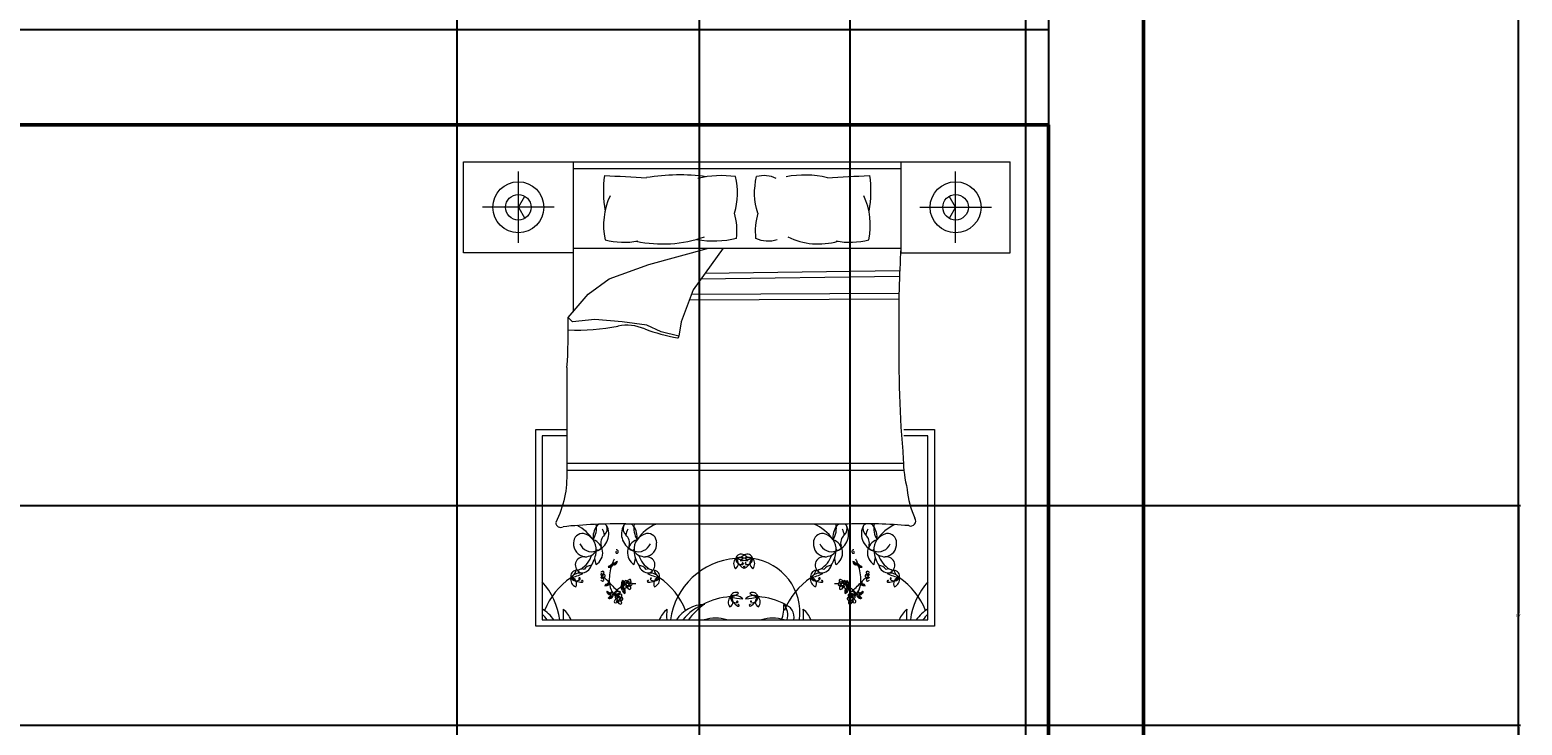
# Model space of a CAD drawing. Units: inches. Extents: x 3 to 576, y -689 to 51.
# Tile 11 of 21: x 435 to 576, y -506 to -440. Entities that reach past the tile are written whole.
import ezdxf

# ---------------------------------------------------------------- set-up
doc = ezdxf.new("R2010")
doc.units = ezdxf.units.IN
doc.header["$MEASUREMENT"] = 0
for name, color, linetype, lineweight in [('A-ANNO-DIMS', 2, 'Continuous', 18), ('A-FURN', 8, 'Continuous', 18), ('A-WALL', 7, 'Continuous', 50)]:
    doc.layers.add(name, color=color, linetype=linetype, lineweight=lineweight)
doc.styles.get("Standard").update_dxf_attribs({"font": 'arial.ttf'})
doc.dimstyles.get("Standard").update_dxf_attribs({"dimtxt": 0.18, "dimasz": 0.18, "dimexe": 0.18, "dimexo": 0.0625, "dimgap": 0.09, "dimtad": 0, "dimtih": 1, "dimtoh": 1, "dimdec": 0, "dimzin": 0, "dimdsep": 46, "dimlunit": 3, "dimtxsty": 'Standard', "dimcen": 0.09, "dimadec": 0, "dimazin": 0, "dimtfac": 1, "dimtdec": 0, "dimtofl": 0, "dimtmove": 0, "dimatfit": 3, "dimfxl": 1, "dimtolj": 1, "dimtzin": 0, "dimarcsym": 0})

# ---------------------------------------------------------------- blocks, each defined once
blk = doc.blocks.new('*D39')
at = {"layer": 'A-ANNO-DIMS', "color": 0, "lineweight": -2, "transparency": 16777216}
for p, q in [((540.36, 15.69), (575.92, 15.69)), ((575.74, 15.51), (575.74, -318.63)), ((575.74, -653.13), (575.74, -318.99)), ((540.36, -653.31), (575.92, -653.31))]:
    blk.add_line(p, q, dxfattribs=at)
at = {"layer": 'A-ANNO-DIMS', "color": 0, "transparency": 16777216}
for points in [[(575.71, 15.51), (575.77, 15.51), (575.74, 15.69)], [(575.71, -653.13), (575.77, -653.13), (575.74, -653.31)]]:
    blk.add_solid(points, dxfattribs=at)
at = {"layer": 'Defpoints', "color": 0, "transparency": 16777216}
for p in [(540.29, 15.69), (540.29, -653.31), (575.74, -653.31)]:
    blk.add_point(p, dxfattribs=at)
at = {"layer": 'A-ANNO-DIMS', "color": 0, "transparency": 16777216, "insert": (575.74, -318.81), "char_height": 0.18, "attachment_point": 5}
blk.add_mtext('\\A1;55\'-9"', dxfattribs=at)
blk = doc.blocks.new('*D71')
at = {"layer": 'A-ANNO-DIMS', "color": 0, "lineweight": -2, "transparency": 16777216}
for p, q in [((531.23, -368.31), (2.66, -368.31)), ((2.84, -368.49), (2.84, -404.13)), ((2.84, -440.13), (2.84, -404.49)), ((531.23, -440.31), (2.66, -440.31))]:
    blk.add_line(p, q, dxfattribs=at)
at = {"layer": 'A-ANNO-DIMS', "color": 0, "transparency": 16777216}
for points in [[(2.81, -368.49), (2.87, -368.49), (2.84, -368.31)], [(2.81, -440.13), (2.87, -440.13), (2.84, -440.31)]]:
    blk.add_solid(points, dxfattribs=at)
at = {"layer": 'Defpoints', "color": 0, "transparency": 16777216}
for p in [(531.29, -368.31), (2.84, -440.31), (531.29, -440.31)]:
    blk.add_point(p, dxfattribs=at)
at = {"layer": 'A-ANNO-DIMS', "color": 0, "transparency": 16777216, "insert": (2.84, -404.31), "char_height": 0.18, "attachment_point": 5}
blk.add_mtext('\\A1;6\'-0"', dxfattribs=at)
blk = doc.blocks.new('*D72')
at = {"layer": 'A-ANNO-DIMS', "color": 0, "lineweight": -2, "transparency": 16777216}
for p, q in [((531.23, -440.31), (2.66, -440.31)), ((2.84, -440.49), (2.84, -444.63)), ((2.84, -449.13), (2.84, -444.99)), ((531.23, -449.31), (2.66, -449.31))]:
    blk.add_line(p, q, dxfattribs=at)
at = {"layer": 'A-ANNO-DIMS', "color": 0, "transparency": 16777216}
for points in [[(2.81, -440.49), (2.87, -440.49), (2.84, -440.31)], [(2.81, -449.13), (2.87, -449.13), (2.84, -449.31)]]:
    blk.add_solid(points, dxfattribs=at)
at = {"layer": 'Defpoints', "color": 0, "transparency": 16777216}
for p in [(531.29, -440.31), (2.84, -449.31), (531.29, -449.31)]:
    blk.add_point(p, dxfattribs=at)
at = {"layer": 'A-ANNO-DIMS', "color": 0, "transparency": 16777216, "insert": (2.84, -444.81), "char_height": 0.18, "attachment_point": 5}
blk.add_mtext('\\A1;0\'-9"', dxfattribs=at)
blk = doc.blocks.new('*D73')
at = {"layer": 'A-ANNO-DIMS', "color": 0, "lineweight": -2, "transparency": 16777216}
for p, q in [((531.23, -449.31), (2.66, -449.31)), ((2.84, -449.49), (2.84, -518.13)), ((2.84, -587.13), (2.84, -518.49)), ((531.23, -587.31), (2.66, -587.31))]:
    blk.add_line(p, q, dxfattribs=at)
at = {"layer": 'A-ANNO-DIMS', "color": 0, "transparency": 16777216}
for points in [[(2.81, -449.49), (2.87, -449.49), (2.84, -449.31)], [(2.81, -587.13), (2.87, -587.13), (2.84, -587.31)]]:
    blk.add_solid(points, dxfattribs=at)
at = {"layer": 'Defpoints', "color": 0, "transparency": 16777216}
for p in [(531.29, -449.31), (2.84, -587.31), (531.29, -587.31)]:
    blk.add_point(p, dxfattribs=at)
at = {"layer": 'A-ANNO-DIMS', "color": 0, "transparency": 16777216, "insert": (2.84, -518.31), "char_height": 0.18, "attachment_point": 5}
blk.add_mtext('\\A1;11\'-6"', dxfattribs=at)
blk = doc.blocks.new('*D77')
at = {"layer": 'A-ANNO-DIMS', "color": 0, "lineweight": -2, "transparency": 16777216}
for p, q in [((372.29, -263.37), (372.29, -688.94)), ((531.29, -263.37), (531.29, -688.94)), ((372.47, -688.76), (451.4, -688.76)), ((531.11, -688.76), (452.18, -688.76))]:
    blk.add_line(p, q, dxfattribs=at)
at = {"layer": 'A-ANNO-DIMS', "color": 0, "transparency": 16777216}
for points in [[(372.47, -688.73), (372.47, -688.79), (372.29, -688.76)], [(531.11, -688.73), (531.11, -688.79), (531.29, -688.76)]]:
    blk.add_solid(points, dxfattribs=at)
at = {"layer": 'Defpoints', "color": 0, "transparency": 16777216}
for p in [(372.29, -263.31), (531.29, -263.31), (531.29, -688.76)]:
    blk.add_point(p, dxfattribs=at)
at = {"layer": 'A-ANNO-DIMS', "color": 0, "transparency": 16777216, "insert": (451.79, -688.76), "char_height": 0.18, "attachment_point": 5}
blk.add_mtext('\\A1;13\'-3"', dxfattribs=at)
blk = doc.blocks.new('*D82')
at = {"layer": 'A-ANNO-DIMS', "color": 0, "lineweight": -2, "transparency": 16777216}
for p, q in [((395.37, -359.37), (395.37, -688.94)), ((475.37, -359.37), (475.37, -688.94)), ((395.55, -688.76), (435.04, -688.76)), ((475.19, -688.76), (435.7, -688.76))]:
    blk.add_line(p, q, dxfattribs=at)
at = {"layer": 'A-ANNO-DIMS', "color": 0, "transparency": 16777216}
for points in [[(395.55, -688.73), (395.55, -688.79), (395.37, -688.76)], [(475.19, -688.73), (475.19, -688.79), (475.37, -688.76)]]:
    blk.add_solid(points, dxfattribs=at)
at = {"layer": 'Defpoints', "color": 0, "transparency": 16777216}
for p in [(395.37, -359.31), (475.37, -359.31), (475.37, -688.76)]:
    blk.add_point(p, dxfattribs=at)
at = {"layer": 'A-ANNO-DIMS', "color": 0, "transparency": 16777216, "insert": (435.37, -688.76), "char_height": 0.18, "attachment_point": 5}
blk.add_mtext('\\A1;6\'-8"', dxfattribs=at)
blk = doc.blocks.new('*D83')
at = {"layer": 'A-ANNO-DIMS', "color": 0, "lineweight": -2, "transparency": 16777216}
for p, q in [((475.37, -359.37), (475.37, -688.94)), ((531.29, -359.37), (531.29, -688.94)), ((475.55, -688.76), (503, -688.76)), ((531.11, -688.76), (503.66, -688.76))]:
    blk.add_line(p, q, dxfattribs=at)
at = {"layer": 'A-ANNO-DIMS', "color": 0, "transparency": 16777216}
for points in [[(475.55, -688.73), (475.55, -688.79), (475.37, -688.76)], [(531.11, -688.73), (531.11, -688.79), (531.29, -688.76)]]:
    blk.add_solid(points, dxfattribs=at)
at = {"layer": 'Defpoints', "color": 0, "transparency": 16777216}
for p in [(475.37, -359.31), (531.29, -359.31), (531.29, -688.76)]:
    blk.add_point(p, dxfattribs=at)
at = {"layer": 'A-ANNO-DIMS', "color": 0, "transparency": 16777216, "insert": (503.33, -688.76), "char_height": 0.18, "attachment_point": 5}
blk.add_mtext('\\A1;4\'-8"', dxfattribs=at)
blk = doc.blocks.new('*D97')
at = {"layer": 'A-ANNO-DIMS', "color": 0, "lineweight": -2, "transparency": 16777216}
for p, q in [((424.15, -506.1), (575.92, -506.1)), ((575.74, -506.28), (575.74, -546.52)), ((575.74, -587.13), (575.74, -546.89)), ((424.15, -587.31), (575.92, -587.31))]:
    blk.add_line(p, q, dxfattribs=at)
at = {"layer": 'A-ANNO-DIMS', "color": 0, "transparency": 16777216}
for points in [[(575.71, -506.28), (575.77, -506.28), (575.74, -506.1)], [(575.71, -587.13), (575.77, -587.13), (575.74, -587.31)]]:
    blk.add_solid(points, dxfattribs=at)
at = {"layer": 'Defpoints', "color": 0, "transparency": 16777216}
for p in [(424.09, -506.1), (424.09, -587.31), (575.74, -587.31)]:
    blk.add_point(p, dxfattribs=at)
at = {"layer": 'A-ANNO-DIMS', "color": 0, "transparency": 16777216, "insert": (575.74, -546.71), "char_height": 0.18, "attachment_point": 5}
blk.add_mtext('\\A1;6\'-9"', dxfattribs=at)
blk = doc.blocks.new('*D103')
at = {"layer": 'A-ANNO-DIMS', "color": 0, "lineweight": -2, "transparency": 16777216}
for p, q in [((498.29, -50.37), (498.29, -688.94)), ((531.29, -50.37), (531.29, -688.94)), ((498.47, -688.76), (514.46, -688.76)), ((531.11, -688.76), (515.12, -688.76))]:
    blk.add_line(p, q, dxfattribs=at)
at = {"layer": 'A-ANNO-DIMS', "color": 0, "transparency": 16777216}
for points in [[(498.47, -688.73), (498.47, -688.79), (498.29, -688.76)], [(531.11, -688.73), (531.11, -688.79), (531.29, -688.76)]]:
    blk.add_solid(points, dxfattribs=at)
at = {"layer": 'Defpoints', "color": 0, "transparency": 16777216}
for p in [(498.29, -50.31), (531.29, -50.31), (531.29, -688.76)]:
    blk.add_point(p, dxfattribs=at)
at = {"layer": 'A-ANNO-DIMS', "color": 0, "transparency": 16777216, "insert": (514.79, -688.76), "char_height": 0.18, "attachment_point": 5}
blk.add_mtext('\\A1;2\'-9"', dxfattribs=at)
blk = doc.blocks.new('*D111')
at = {"layer": 'A-ANNO-DIMS', "color": 0, "lineweight": -2, "transparency": 16777216}
for p, q in [((397.08, -485.31), (575.92, -485.31)), ((575.74, -485.49), (575.74, -495.52)), ((575.74, -505.92), (575.74, -495.89)), ((397.08, -506.1), (575.92, -506.1))]:
    blk.add_line(p, q, dxfattribs=at)
at = {"layer": 'A-ANNO-DIMS', "color": 0, "transparency": 16777216}
for points in [[(575.71, -485.49), (575.77, -485.49), (575.74, -485.31)], [(575.71, -505.92), (575.77, -505.92), (575.74, -506.1)]]:
    blk.add_solid(points, dxfattribs=at)
at = {"layer": 'Defpoints', "color": 0, "transparency": 16777216}
for p in [(397.02, -485.31), (397.02, -506.1), (575.74, -506.1)]:
    blk.add_point(p, dxfattribs=at)
at = {"layer": 'A-ANNO-DIMS', "color": 0, "transparency": 16777216, "insert": (575.74, -495.71), "char_height": 0.18, "attachment_point": 5}
blk.add_mtext('\\A1;1\'-9"', dxfattribs=at)
blk = doc.blocks.new('*D126')
at = {"layer": 'A-ANNO-DIMS', "color": 0, "lineweight": -2, "transparency": 16777216}
for p, q in [((512.51, -386.37), (512.51, -688.94)), ((529.12, -391.8), (529.12, -688.94)), ((512.69, -688.76), (520.28, -688.76)), ((528.94, -688.76), (521.35, -688.76))]:
    blk.add_line(p, q, dxfattribs=at)
at = {"layer": 'A-ANNO-DIMS', "color": 0, "transparency": 16777216}
for points in [[(512.69, -688.73), (512.69, -688.79), (512.51, -688.76)], [(528.94, -688.73), (528.94, -688.79), (529.12, -688.76)]]:
    blk.add_solid(points, dxfattribs=at)
at = {"layer": 'Defpoints', "color": 0, "transparency": 16777216}
for p in [(512.51, -386.31), (529.12, -391.74), (529.12, -688.76)]:
    blk.add_point(p, dxfattribs=at)
at = {"layer": 'A-ANNO-DIMS', "color": 0, "transparency": 16777216, "insert": (520.82, -688.76), "char_height": 0.18, "attachment_point": 5}
blk.add_mtext('\\A1;1\'-4 1/2"', dxfattribs=at)

msp = doc.modelspace()

# ---------------------------------------------------------------- linework, layer by layer
at = {"layer": 'A-FURN'}
for p, q in [((476.01, -452.8), (527.69, -452.8)), ((486.35, -452.8), (486.35, -466.98)), ((481.18, -460.48), (481.18, -453.73)), ((517.35, -453.46), (486.35, -453.46)), ((522.52, -460.48), (522.52, -453.73)), ((484.56, -457.1), (477.8, -457.1)), ((519.15, -457.1), (525.9, -457.1)), ((486.35, -460.96), (517.35, -460.96)), ((493.53, -462.5), (499.16, -460.96)), ((500.54, -460.96), (497.71, -464.9)), ((489.76, -463.86), (493.53, -462.5)), ((487.77, -465.32), (489.76, -463.86)), ((517.2, -463.64), (498.43, -463.9)), ((517.22, -463.11), (498.82, -463.37)), ((485.89, -467.52), (487.77, -465.32)), ((497.71, -464.9), (496.56, -467.94)), ((517.17, -465.27), (497.55, -465.34)), ((517.17, -465.8), (497.34, -465.88)), ((486.3, -467.94), (485.89, -467.52)), ((488.4, -467.73), (486.3, -467.94)), ((491.01, -467.94), (488.4, -467.73)), ((493.32, -468.25), (491.01, -467.94)), ((494.68, -468.88), (493.32, -468.25)), ((496.56, -467.94), (496.35, -469.3)), ((496.35, -469.3), (494.68, -468.88)), ((482.83, -478.13), (485.76, -478.13)), ((482.83, -496.74), (482.83, -478.13)), ((517.64, -478.13), (520.51, -478.13)), ((520.51, -478.13), (520.51, -496.74)), ((485.76, -478.73), (483.43, -478.73)), ((483.43, -478.73), (483.43, -496.14)), ((519.91, -478.73), (517.63, -478.73)), ((519.91, -496.14), (519.91, -478.73)), ((517.59, -481.35), (485.75, -481.35)), ((517.64, -482), (485.75, -482)), ((512.34, -487.07), (491.36, -487.07)), ((488.53, -490.91), (488.41, -490.32)), ((492.14, -490.91), (492.25, -490.32)), ((511.21, -490.91), (511.09, -490.32)), ((514.82, -490.91), (514.93, -490.32)), ((483.43, -496.14), (519.91, -496.14)), ((520.51, -496.74), (482.83, -496.74))]:
    msp.add_line(p, q, dxfattribs=at)
for points in [[(486.35, -461.41), (476.01, -461.41), (476.01, -452.8)], [(517.35, -452.8), (517.35, -461.41), (527.69, -461.41), (527.69, -452.8)], [(481.18, -457.1), (481.78, -456.06)], [(481.18, -457.1), (481.78, -458.15)], [(522.52, -457.1), (521.92, -456.06)], [(522.52, -457.1), (521.92, -458.15)]]:
    msp.add_lwpolyline(points, dxfattribs=at)
for points in [[(489.32, -454.08, 0.074897), (489.38, -457.46, -0.472817)], [(501.61, -457.65, 0.14099), (501.71, -454.2, 0.235245)], [(503.82, -457.65, -0.14099), (503.71, -454.2, -0.235245)], [(514.39, -454.08, -0.074897), (514.32, -457.46, 0.472817)], [(485.78, -472.25, 0.001242), (485.75, -482.06, -0.127202), (484.72, -486.94)], [(517.57, -480.94, 0.056112), (517.95, -483.79, 0.095341), (518.68, -486.53)]]:
    msp.add_lwpolyline(points, format="xyb", dxfattribs=at)
for centre, radius in [((481.18, -457.1), 2.41), ((522.52, -457.1), 2.41), ((481.18, -457.1), 1.21), ((522.52, -457.1), 1.21), ((491.51, -492.78), 0.132), ((511.83, -492.78), 0.132), ((490.65, -494.16), 0.132), ((512.69, -494.16), 0.132)]:
    msp.add_circle(centre, radius, dxfattribs=at)
for centre, radius, start, end in [((517.8, 37.7), 492.61, 266.6852, 267.1498), ((496.4, -472.78), 18.74, 82.2196, 99.497), ((500.36, -463.31), 9.21, 81.5249, 103.96), ((504.42, -456.66), 2.56, 63.3437, 106.1026), ((508.25, -463.13), 9.08, 76.3427, 101.1841), ((485.9, 37.7), 492.61, 272.8502, 273.3148), ((495.9, -458.81), 6.66, 155.1316, 191.7583), ((507.8, -458.81), 6.66, 348.2417, 24.8684), ((495.52, -459.38), 6.33, 354.0129, 15.8293), ((509.91, -459.38), 6.33, 164.1707, 185.9871), ((494.81, -448.56), 12.01, 258.0397, 289.2615), ((509.55, -453.99), 6.58, 243.8761, 286.1746), ((491.16, -453.48), 6.93, 255.1039, 281.0369), ((499.67, -451.18), 9.11, 259.8617, 283.6238), ((504.77, -457.55), 2.74, 245.0183, 288.5407), ((512.54, -453.48), 6.93, 258.9631, 284.8961), ((609.99, -467.28), 92.85, 176.1, 180.9282), ((438.5, -468.8), 47.4, 355.8294, 1.553), ((486.77, -449.22), 19.5, 267.4519, 281.3392), ((491.43, -472.47), 4.21, 66.2616, 101.3392), ((499.94, -449.77), 20.04, 250.1194, 259.3383), ((496.23, -469.34), 0.125, 268.8623, 19.7536), ((638.26, -470.65), 121.12, 179.1145, 184.8735), ((518.28, -486.79), 0.471, 246.5219, 33.8264), ((485.19, -486.91), 0.477, 183.98, 297.3412), ((490.74, -540.86), 53.8, 89.3433, 95.6887), ((487.27, -488.83), 0.872, 84.4856, 181.0538), ((484.99, -490.71), 3.91, 33.6671, 63.2997), ((487, -489.48), 1.55, 355.2933, 76.921), ((490.23, -488.38), 1.99, 145.785, 184.7304), ((486.43, -487.45), 2.14, 328.8218, 9.1554), ((489.08, -487.64), 0.622, 120.0293, 142.325), ((488.08, -488.01), 1.65, 289.2822, 29.1751), ((490.03, -488.89), 1.06, 131.5653, 195.1471), ((487.84, -488.31), 1.49, 7.436, 29.9149), ((488.81, -487.52), 0.773, 311.5653, 23.8354), ((489.08, -487.64), 0.622, 44.4517, 63.558), ((492.58, -488.01), 1.65, 150.8249, 250.7178), ((491.85, -487.52), 0.773, 156.1646, 228.4347), ((491.58, -487.64), 0.622, 113.229, 135.5483), ((490.63, -488.89), 1.06, 344.8529, 48.4347), ((492.83, -488.31), 1.49, 150.0851, 172.564), ((491.58, -487.64), 0.622, 37.675, 66.7144), ((490.43, -488.38), 1.99, 355.2696, 34.215), ((494.24, -487.45), 2.14, 169.7133, 211.1782), ((493.66, -489.48), 1.55, 103.079, 184.7067), ((495.67, -490.71), 3.91, 111.4941, 146.3329), ((493.39, -488.83), 0.872, 358.9462, 95.5144), ((509.95, -488.83), 0.872, 84.4856, 181.0538), ((507.67, -490.71), 3.91, 33.6671, 68.5059), ((509.68, -489.48), 1.55, 355.2933, 76.921), ((512.91, -488.38), 1.99, 145.785, 184.7304), ((509.11, -487.45), 2.14, 328.8218, 10.2867), ((511.76, -487.64), 0.622, 113.2856, 142.325), ((510.76, -488.01), 1.65, 289.2822, 29.1751), ((512.71, -488.89), 1.06, 131.5653, 195.1471), ((510.52, -488.31), 1.49, 7.436, 29.9149), ((511.76, -487.64), 0.622, 44.4517, 66.7144), ((511.49, -487.52), 0.773, 311.5653, 23.8354), ((513.92, -537.33), 50.28, 85.2402, 91.8035), ((515.26, -488.01), 1.65, 150.8249, 250.7178), ((514.53, -487.52), 0.773, 156.1646, 228.4347), ((514.26, -487.64), 0.622, 106.6343, 135.5483), ((513.31, -488.89), 1.06, 344.8529, 48.4347), ((515.51, -488.31), 1.49, 150.0851, 172.564), ((514.26, -487.64), 0.622, 37.675, 72.5814), ((513.11, -488.38), 1.99, 355.2696, 34.215), ((516.92, -487.45), 2.14, 169.249, 211.1782), ((516.34, -489.48), 1.55, 103.079, 184.7067), ((518.35, -490.71), 3.91, 113.6453, 146.3329), ((516.07, -488.83), 0.872, 358.9462, 95.5144), ((487.63, -488.96), 1.23, 174.9449, 262.8857), ((488.11, -488.49), 1.2, 201.5819, 291.4221), ((487.41, -488.68), 1.5, 272.3591, 324.0401), ((487.88, -489.79), 1.28, 299.9085, 73.1337), ((490.23, -488.38), 1.99, 212.7011, 216.3445), ((488.7, -489.25), 0.321, 257.3041, 15.1471), ((490.47, -489.68), 0.162, 280.4384, 100.4136), ((492.78, -489.79), 1.28, 106.8663, 240.0915), ((491.96, -489.25), 0.321, 164.8529, 282.6959), ((490.43, -488.38), 1.99, 323.6555, 327.2989), ((493.25, -488.68), 1.5, 215.9599, 267.6409), ((492.55, -488.49), 1.2, 248.5779, 338.4181), ((493.03, -488.96), 1.23, 277.1143, 5.0551), ((510.31, -488.96), 1.23, 174.9449, 262.8857), ((510.79, -488.49), 1.2, 201.5819, 291.4221), ((510.09, -488.68), 1.5, 272.3591, 324.0401), ((510.56, -489.79), 1.28, 299.9085, 73.1337), ((512.91, -488.38), 1.99, 212.7011, 216.3445), ((511.38, -489.25), 0.321, 257.3041, 15.1471), ((512.87, -489.68), 0.162, 79.5864, 259.5616), ((515.46, -489.79), 1.28, 106.8663, 240.0915), ((514.64, -489.25), 0.321, 164.8529, 282.6959), ((513.11, -488.38), 1.99, 323.6555, 327.2989), ((515.93, -488.68), 1.5, 215.9599, 267.6409), ((515.23, -488.49), 1.2, 248.5779, 338.4181), ((515.71, -488.96), 1.23, 277.1143, 5.0551), ((487.34, -490.95), 0.776, 80.264, 250.8688), ((485.81, -489.24), 2.44, 301.2614, 341.7045), ((487.16, -490.71), 0.968, 265.969, 344.3045), ((488.2, -492), 1.03, 96.1662, 141.5825), ((485.78, -489.44), 2.77, 326.2883, 356.5076), ((489.34, -490.36), 0.83, 308.2101, 316.3071), ((489.85, -490.9), 0.248, 278.3432, 4.2869), ((489.71, -490.69), 0.433, 300.656, 332.6341), ((490.04, -490.97), 0.105, 55.7657, 157.4417), ((494.06, -492.34), 4.28, 153.0032, 159.8941), ((490.2, -490.88), 0.105, 84.3784, 186.0543), ((490.1, -490.45), 0.433, 269.1859, 301.164), ((490.23, -490.68), 0.248, 237.5332, 323.4768), ((489.99, -489.97), 0.83, 285.5129, 293.6099), ((490.53, -490.9), 0.271, 87.3579, 140.4944), ((489.91, -490.12), 0.817, 301.164, 321.5612), ((490.48, -489.74), 0.0996, 102.7051, 280.4384), ((489.24, -489.98), 1.46, 324.6898, 333.4936), ((494.88, -489.44), 2.77, 183.4924, 213.7117), ((494.86, -489.24), 2.44, 198.2955, 238.7386), ((492.46, -492), 1.03, 38.4175, 83.8338), ((493.5, -490.71), 0.968, 195.6955, 274.031), ((493.32, -490.95), 0.776, 289.1312, 99.736), ((502.25, -497.05), 6.75, 94.4623, 172.255), ((502.28, -490.83), 0.748, 137.7873, 219.1145), ((501.43, -490.81), 0.564, 298.5391, 58.3627), ((502.27, -490.48), 0.559, 63.0274, 163.8037), ((501.7, -489.17), 1.15, 271.4585, 315.3727), ((502.17, -491.3), 1.07, 45.5411, 114.3101), ((503.14, -485.82), 4.72, 252.593, 267.2582), ((502.28, -490.35), 0.552, 177.7585, 283.852), ((503.34, -489.77), 1.71, 198.9159, 238.011), ((502.9, -491.3), 1.07, 65.6899, 134.4589), ((501.92, -485.82), 4.72, 272.7418, 287.407), ((502.39, -490.81), 0.073, 283.852, 219.9245), ((502.8, -490.48), 0.559, 16.1963, 116.9726), ((503.37, -489.17), 1.15, 224.6273, 268.5415), ((502.66, -490.78), 0.044, 320.1909, 256.0209), ((501.72, -489.77), 1.71, 301.989, 341.0841), ((502.78, -490.35), 0.552, 256.148, 2.2415), ((503.63, -490.81), 0.564, 121.6373, 241.4609), ((502.78, -490.83), 0.748, 320.8855, 42.2127), ((502.59, -495.5), 5.22, 352.8636, 81.8197), ((510.02, -490.95), 0.776, 80.264, 250.8688), ((508.49, -489.24), 2.44, 301.2614, 341.7045), ((509.84, -490.71), 0.968, 265.969, 344.3045), ((510.88, -492), 1.03, 96.1662, 141.5825), ((508.46, -489.44), 2.77, 326.2883, 356.5076), ((513.44, -490.12), 0.817, 218.4388, 238.836), ((512.81, -490.9), 0.271, 39.5056, 92.6421), ((514.1, -489.98), 1.46, 206.5064, 215.3102), ((512.86, -489.74), 0.0996, 259.5616, 77.2949), ((513.11, -490.68), 0.248, 216.5232, 302.4668), ((513.24, -490.45), 0.433, 238.836, 270.8141), ((513.35, -489.97), 0.83, 246.3901, 254.4871), ((509.28, -492.34), 4.28, 20.1059, 26.9968), ((513.14, -490.88), 0.105, 353.9457, 95.6216), ((513.3, -490.97), 0.105, 22.5583, 124.2343), ((513.49, -490.9), 0.248, 175.7131, 261.6568), ((513.63, -490.69), 0.433, 207.3659, 239.344), ((514, -490.36), 0.83, 223.6929, 231.7899), ((517.56, -489.44), 2.77, 183.4924, 213.7117), ((517.54, -489.24), 2.44, 198.2955, 238.7386), ((516.18, -490.71), 0.968, 195.6955, 274.031), ((515.14, -492), 1.03, 38.4175, 83.8338), ((516, -490.95), 0.776, 289.1312, 99.736), ((489.95, -497.72), 6.75, 124.3865, 158.5908), ((486.69, -492.02), 0.559, 92.9516, 193.728), ((486.87, -492.31), 0.748, 167.7115, 249.0387), ((485.54, -491.17), 1.15, 301.3827, 345.2969), ((487.01, -492.78), 1.07, 75.4653, 144.2343), ((485.12, -487.54), 4.72, 282.5173, 297.1824), ((486.13, -492.72), 0.564, 328.4633, 88.2869), ((487.27, -490.87), 1.71, 228.8402, 267.9352), ((486.63, -491.9), 0.552, 207.6827, 313.7762), ((487.18, -491.79), 0.475, 63.9755, 143.2681), ((486.96, -492.24), 0.073, 313.7762, 249.7183), ((489.14, -491.79), 0.22, 101.5637, 142.6358), ((488.96, -492), 0.132, 273.2768, 86.7232), ((489.14, -492.24), 0.217, 217.7621, 259.0403), ((489.11, -491.87), 0.126, 91.1081, 181.8675), ((489.37, -491.95), 0.4, 203.4276, 227.6104), ((489.25, -492.12), 0.272, 80.3487, 133.6538), ((489.2, -491.9), 0.215, 229.7889, 317.6792), ((488.97, -491.62), 0.316, 288.7263, 352.5032), ((488.95, -492.35), 0.306, 355.053, 68.3618), ((489.19, -492.41), 0.431, 83.0852, 105.7171), ((489.18, -491.64), 0.102, 345.2356, 144.9248), ((489.16, -492.37), 0.101, 232.4737, 355.053), ((486.21, -495.98), 4.91, 43.1541, 52.0459), ((489.27, -491.97), 0.113, 317.6792, 80.3487), ((489.91, -491.28), 0.271, 101.3256, 154.4621), ((489.52, -490.36), 0.817, 280.2588, 300.656), ((489.71, -489.7), 1.46, 268.3264, 277.1302), ((494.06, -492.34), 4.28, 163.5842, 183.8277), ((491.69, -492.57), 0.22, 101.5637, 176.365), ((491.73, -492.42), 0.102, 345.2356, 144.9248), ((493.48, -491.79), 0.475, 36.7319, 116.0245), ((493.65, -492.78), 1.07, 35.7657, 104.5347), ((495.54, -487.54), 4.72, 242.8176, 257.4827), ((493.4, -490.87), 1.71, 272.0648, 311.1598), ((494.03, -491.9), 0.552, 226.2238, 332.3173), ((493.71, -492.21), 0.044, 290.2667, 226.2271), ((494.54, -492.72), 0.564, 91.7131, 211.5367), ((493.98, -492.02), 0.559, 346.272, 87.0484), ((495.12, -491.17), 1.15, 194.7031, 238.6173), ((493.79, -492.31), 0.748, 290.9613, 12.2885), ((490.71, -497.72), 6.75, 21.4092, 55.6135), ((502.48, -491.15), 0.0838, 238.011, 71.5592), ((502.5, -491.11), 0.0407, 71.5592, 188.0167), ((502.58, -491.15), 0.0838, 108.4408, 301.989), ((502.57, -491.11), 0.0407, 351.9833, 108.4408), ((512.63, -497.72), 6.75, 124.3865, 158.5908), ((509.37, -492.02), 0.559, 92.9516, 193.728), ((509.55, -492.31), 0.748, 167.7115, 249.0387), ((508.22, -491.17), 1.15, 301.3827, 345.2969), ((509.69, -492.78), 1.07, 75.4653, 144.2343), ((507.8, -487.54), 4.72, 282.5173, 297.1824), ((509.31, -491.9), 0.552, 207.6827, 313.7762), ((509.95, -490.87), 1.71, 228.8402, 267.9352), ((508.81, -492.72), 0.564, 328.4633, 88.2869), ((509.86, -491.79), 0.475, 63.9755, 143.2681), ((509.64, -492.24), 0.073, 313.7762, 249.7183), ((511.61, -492.42), 0.102, 35.0752, 194.7644), ((511.65, -492.57), 0.22, 3.635, 78.4363), ((509.28, -492.34), 4.28, 356.1723, 16.4158), ((513.82, -490.36), 0.817, 239.344, 259.7412), ((513.64, -489.7), 1.46, 262.8698, 271.6736), ((513.43, -491.28), 0.271, 25.5379, 78.6744), ((517.13, -495.98), 4.91, 127.9541, 136.8459), ((514.07, -491.97), 0.113, 99.6513, 222.3208), ((514.14, -491.9), 0.215, 222.3208, 310.2111), ((514.1, -492.12), 0.272, 46.3462, 99.6513), ((514.16, -491.64), 0.102, 35.0752, 194.7644), ((514.38, -491.62), 0.316, 187.4968, 251.2737), ((514.39, -492.35), 0.306, 111.6382, 184.947), ((514.18, -492.37), 0.101, 184.947, 307.5263), ((514.15, -492.41), 0.431, 74.2829, 96.9148), ((514.23, -491.87), 0.126, 358.1325, 88.8919), ((514.2, -491.79), 0.22, 37.3642, 78.4363), ((513.97, -491.95), 0.4, 312.3896, 336.5724), ((514.2, -492.24), 0.217, 280.9597, 322.2379), ((514.38, -492), 0.132, 93.2768, 266.7232), ((516.16, -491.79), 0.475, 36.7319, 116.0245), ((516.33, -492.78), 1.07, 35.7657, 104.5347), ((518.22, -487.54), 4.72, 242.8176, 257.4827), ((516.08, -490.87), 1.71, 272.0648, 311.1598), ((516.71, -491.9), 0.552, 226.2238, 332.3173), ((516.39, -492.21), 0.044, 290.2667, 226.2271), ((517.22, -492.72), 0.564, 91.7131, 211.5367), ((517.8, -491.17), 1.15, 194.7031, 238.6173), ((516.66, -492.02), 0.559, 346.272, 87.0484), ((516.47, -492.31), 0.748, 290.9613, 12.2885), ((513.39, -497.72), 6.75, 21.4092, 55.6135), ((478.41, -497.05), 6.75, 7.745, 41.8856), ((487.2, -492.45), 0.0407, 101.4834, 217.9409), ((487.21, -492.49), 0.0838, 267.9352, 101.4834), ((489.6, -493.02), 0.271, 101.3256, 154.4621), ((489.21, -492.1), 0.817, 280.2588, 300.656), ((489.4, -491.44), 1.46, 268.3264, 277.1302), ((489.03, -492.1), 0.83, 308.2101, 316.3071), ((489.69, -493.49), 0.147, 146.8636, 236.9021), ((491.76, -490.26), 3.84, 235.1882, 238.8844), ((489.94, -493.28), 0.398, 199.4799, 267.6828), ((489.54, -492.64), 0.248, 278.3432, 4.2869), ((489.9, -493.43), 0.343, 212.8155, 277.3992), ((489.73, -492.71), 0.105, 55.7657, 157.4417), ((489.41, -492.43), 0.433, 300.656, 332.6341), ((489.86, -493.42), 0.152, 238.8844, 314.2646), ((491.93, -492.45), 2.15, 184.756, 209.2041), ((495.02, -487.88), 7.06, 222.2412, 232.1744), ((489.82, -493.76), 0.343, 280.3057, 17.1958), ((489.79, -493.79), 0.152, 306.3746, 21.7548), ((490.04, -493.69), 0.115, 19.3605, 201.7548), ((490.04, -493.61), 0.115, 311.8703, 134.2646), ((492.2, -494.65), 2.29, 153.7819, 158.2913), ((490.38, -493.09), 0.6, 247.2305, 319.0635), ((490.18, -493.29), 0.353, 264.4544, 310.6188), ((491.93, -492.45), 2.15, 214.0033, 222.4917), ((490.44, -493.43), 0.365, 218.3208, 298.8162), ((492.15, -495.3), 2.57, 120.544, 139.818), ((490.68, -493.88), 0.424, 70.0041, 130.6188), ((490.41, -493.36), 0.436, 297.7043, 344.3516), ((490.83, -493.96), 0.22, 101.5637, 176.365), ((490.87, -493.8), 0.102, 345.2356, 144.9248), ((490.5, -492.58), 0.6, 304.5369, 16.3699), ((490.82, -492.72), 0.365, 272.8499, 356.1226), ((490.57, -492.86), 0.353, 321.7607, 7.9252), ((490.64, -493.37), 0.353, 8.7227, 54.8872), ((490.66, -493.65), 0.6, 0.278, 72.111), ((491.34, -492.75), 0.424, 127.3105, 187.9252), ((490.93, -493.43), 0.365, 20.5253, 88.5375), ((491.41, -493.25), 0.424, 188.7227, 249.3375), ((490.75, -492.7), 0.436, 355.0106, 41.658), ((491.23, -493.02), 0.13, 148.0499, 225.6268), ((492.15, -495.3), 2.57, 113.0501, 113.8477), ((491.48, -493.18), 0.415, 104.7558, 148.0499), ((491.24, -492.88), 0.26, 247.4086, 351.4386), ((491.37, -492.59), 0.179, 126.1046, 271.4281), ((491.35, -492.55), 0.129, 353.7526, 131.7054), ((490.86, -493.46), 0.436, 334.9899, 21.6373), ((491.32, -492.89), 0.0872, 262.906, 7.132), ((491.22, -492.7), 0.181, 0.0645, 61.1507), ((491.27, -492.54), 0.207, 311.8413, 355.7877), ((491.69, -493.02), 0.217, 151.2196, 259.0403), ((491.66, -492.65), 0.126, 91.1081, 181.8675), ((491.92, -492.73), 0.4, 203.4276, 227.6104), ((491.8, -492.91), 0.272, 80.3487, 133.6538), ((491.75, -492.68), 0.215, 229.7889, 317.6792), ((491.52, -492.4), 0.316, 288.7263, 352.5032), ((491.51, -493.14), 0.306, 355.053, 68.3618), ((491.75, -493.19), 0.431, 83.0852, 105.7171), ((491.71, -493.15), 0.101, 232.4737, 355.053), ((491.82, -492.75), 0.113, 317.6792, 80.3487), ((492.15, -495.3), 2.57, 87.1071, 94.7585), ((493.45, -492.49), 0.0838, 78.5166, 272.0648), ((493.46, -492.45), 0.0407, 322.0591, 78.5166), ((501.75, -494.1), 0.559, 63.0274, 163.8037), ((501.18, -492.79), 1.15, 271.4585, 315.3727), ((503.32, -494.1), 0.559, 16.1963, 116.9726), ((503.88, -492.79), 1.15, 224.6273, 268.5415), ((509.88, -492.45), 0.0407, 101.4834, 217.9409), ((509.89, -492.49), 0.0838, 267.9352, 101.4834), ((511.19, -495.3), 2.57, 85.2415, 92.8929), ((511.52, -492.75), 0.113, 99.6513, 222.3208), ((511.59, -492.68), 0.215, 222.3208, 310.2111), ((511.54, -492.91), 0.272, 46.3462, 99.6513), ((511.83, -492.4), 0.316, 187.4968, 251.2737), ((511.84, -493.14), 0.306, 111.6382, 184.947), ((511.63, -493.15), 0.101, 184.947, 307.5263), ((511.6, -493.19), 0.431, 74.2829, 96.9148), ((511.68, -492.65), 0.126, 358.1325, 88.8919), ((511.42, -492.73), 0.4, 312.3896, 336.5724), ((511.65, -493.02), 0.217, 280.9597, 28.7804), ((512.1, -492.88), 0.26, 188.5614, 292.5914), ((512, -492.55), 0.129, 48.2946, 186.2474), ((512.07, -492.54), 0.207, 184.2123, 228.1587), ((512.12, -492.7), 0.181, 118.8493, 179.9355), ((512.03, -492.89), 0.0872, 172.868, 277.094), ((511.98, -492.59), 0.179, 268.5719, 53.8954), ((511.87, -493.18), 0.415, 31.9501, 75.2442), ((512.48, -493.46), 0.436, 158.3627, 205.0101), ((512.41, -493.43), 0.365, 91.4625, 159.4747), ((512.68, -493.65), 0.6, 107.889, 179.722), ((511.93, -493.25), 0.424, 290.6625, 351.2773), ((512.59, -492.7), 0.436, 138.342, 184.9894), ((512.52, -492.72), 0.365, 183.8774, 267.1501), ((511.19, -495.3), 2.57, 66.1523, 66.9499), ((512.11, -493.02), 0.13, 314.3732, 31.9501), ((512.84, -492.58), 0.6, 163.6301, 235.4631), ((512.01, -492.75), 0.424, 352.0748, 52.6895), ((512.7, -493.37), 0.353, 125.1128, 171.2773), ((512.47, -493.8), 0.102, 35.0752, 194.7644), ((512.78, -492.86), 0.353, 172.0748, 218.2393), ((511.19, -495.3), 2.57, 40.182, 59.456), ((512.66, -493.88), 0.424, 49.3812, 109.9959), ((512.97, -493.09), 0.6, 220.9365, 292.7695), ((512.93, -493.36), 0.436, 195.6484, 242.2957), ((512.51, -493.96), 0.22, 3.635, 78.4363), ((508.32, -487.88), 7.06, 307.8256, 317.7588), ((512.91, -493.43), 0.365, 241.1838, 321.6792), ((513.16, -493.29), 0.353, 229.3812, 275.5456), ((511.41, -492.45), 2.15, 317.5083, 325.9967), ((513.3, -493.61), 0.115, 45.7354, 228.1297), ((513.52, -493.76), 0.343, 162.8042, 259.6943), ((513.3, -493.69), 0.115, 338.2452, 160.6395), ((511.14, -494.65), 2.29, 21.7087, 26.2181), ((511.41, -492.45), 2.15, 330.7959, 355.244), ((513.49, -493.42), 0.152, 225.7354, 301.1156), ((513.44, -493.43), 0.343, 262.6008, 327.1845), ((513.55, -493.79), 0.152, 158.2452, 233.6254), ((513.4, -493.28), 0.398, 272.3172, 340.5201), ((513.61, -492.71), 0.105, 22.5583, 124.2343), ((513.8, -492.64), 0.248, 175.7131, 261.6568), ((513.94, -492.43), 0.433, 207.3659, 239.344), ((511.58, -490.26), 3.84, 301.1156, 304.8118), ((514.31, -492.1), 0.83, 223.6929, 231.7899), ((514.13, -492.1), 0.817, 239.344, 259.7412), ((513.65, -493.49), 0.147, 303.0979, 33.1364), ((513.94, -491.44), 1.46, 262.8698, 271.6736), ((513.74, -493.02), 0.271, 25.5379, 78.6744), ((516.13, -492.49), 0.0838, 78.5166, 272.0648), ((516.14, -492.45), 0.0407, 322.0591, 78.5166), ((524.93, -497.05), 6.75, 138.1144, 172.255), ((481.79, -497.96), 3.29, 33.4617, 60.1116), ((483.64, -497.2), 2.74, 22.5547, 48.9546), ((476.12, -495.72), 9.34, 357.4081, 3.6519), ((489.7, -493.66), 0.398, 266.9701, 338.2913), ((487.6, -490.82), 3.84, 302.6784, 306.3746), ((489.8, -493.97), 0.147, 214.3538, 304.3923), ((490.37, -494.41), 0.13, 148.0499, 225.6268), ((490.61, -494.56), 0.415, 104.7558, 148.0499), ((490.38, -494.27), 0.26, 247.4086, 351.4386), ((490.5, -493.98), 0.179, 126.1046, 271.4281), ((490.48, -493.93), 0.129, 353.7526, 131.7054), ((490.45, -494.28), 0.0872, 262.906, 7.132), ((490.36, -494.09), 0.181, 0.0645, 61.1507), ((490.41, -493.93), 0.207, 311.8413, 355.7877), ((490.83, -494.41), 0.217, 151.2196, 259.0403), ((490.8, -494.04), 0.126, 91.1081, 181.8675), ((491.06, -494.12), 0.4, 203.4276, 227.6104), ((490.94, -494.29), 0.272, 80.3487, 133.6538), ((490.89, -494.07), 0.215, 229.7889, 317.6792), ((490.66, -493.79), 0.316, 288.7263, 352.5032), ((490.65, -494.52), 0.306, 355.053, 68.3618), ((490.89, -494.58), 0.431, 83.0852, 105.7171), ((490.85, -494.54), 0.101, 232.4737, 355.053), ((490.96, -494.14), 0.113, 317.6792, 80.3487), ((497.03, -497.2), 2.74, 131.0454, 157.4453), ((504.54, -495.72), 9.34, 176.3481, 182.5919), ((498.87, -497.96), 3.29, 91.272, 146.5383), ((500.05, -498.57), 4.1, 107.8504, 143.6964), ((502.2, -499.72), 6.1, 124.0123, 144.053), ((501.74, -500.67), 6.75, 94.4623, 117.4146), ((501.77, -494.44), 0.748, 137.7873, 219.1145), ((500.92, -494.42), 0.564, 298.5391, 58.3627), ((501.65, -494.91), 1.07, 45.5411, 114.3101), ((502.83, -493.39), 1.71, 198.9159, 238.011), ((502.62, -489.44), 4.72, 252.593, 267.2582), ((501.76, -493.96), 0.552, 177.7585, 283.852), ((501.88, -494.43), 0.073, 283.852, 219.9245), ((501.97, -494.76), 0.0838, 238.011, 71.5592), ((501.98, -494.72), 0.0407, 71.5592, 188.0167), ((503.41, -494.91), 1.07, 65.6899, 134.4589), ((502.44, -489.44), 4.72, 272.7418, 287.407), ((503.1, -494.76), 0.0838, 108.4408, 301.989), ((503.08, -494.72), 0.0407, 351.9833, 108.4408), ((502.24, -493.39), 1.71, 301.989, 341.0841), ((503.18, -494.4), 0.044, 320.1909, 256.0209), ((503.3, -493.96), 0.552, 256.148, 2.2415), ((504.15, -494.42), 0.564, 121.6373, 241.4609), ((503.3, -494.44), 0.748, 320.8855, 42.2127), ((503.33, -500.67), 6.75, 62.5854, 85.5377), ((503.27, -495.02), 3.02, 338.117, 6.6195), ((506.04, -495.86), 1.21, 346.3898, 79.0739), ((505.13, -495.69), 1.53, 342.8609, 41.9049), ((498.8, -495.72), 9.34, 357.4081, 3.6519), ((506.32, -497.2), 2.74, 22.5547, 48.9546), ((512.38, -494.14), 0.113, 99.6513, 222.3208), ((512.45, -494.07), 0.215, 222.3208, 310.2111), ((512.41, -494.29), 0.272, 46.3462, 99.6513), ((512.69, -493.79), 0.316, 187.4968, 251.2737), ((512.7, -494.52), 0.306, 111.6382, 184.947), ((512.49, -494.54), 0.101, 184.947, 307.5263), ((512.46, -494.58), 0.431, 74.2829, 96.9148), ((512.54, -494.04), 0.126, 358.1325, 88.8919), ((512.28, -494.12), 0.4, 312.3896, 336.5724), ((512.51, -494.41), 0.217, 280.9597, 28.7804), ((512.96, -494.27), 0.26, 188.5614, 292.5914), ((512.86, -493.93), 0.129, 48.2946, 186.2474), ((512.94, -493.93), 0.207, 184.2123, 228.1587), ((512.98, -494.09), 0.181, 118.8493, 179.9355), ((512.89, -494.28), 0.0872, 172.868, 277.094), ((512.84, -493.98), 0.179, 268.5719, 53.8954), ((512.73, -494.56), 0.415, 31.9501, 75.2442), ((512.97, -494.41), 0.13, 314.3732, 31.9501), ((513.64, -493.66), 0.398, 201.7087, 273.0299), ((515.74, -490.82), 3.84, 233.6254, 237.3216), ((513.54, -493.97), 0.147, 235.6077, 325.6462), ((519.71, -497.2), 2.74, 131.0454, 157.4453), ((527.22, -495.72), 9.34, 176.3481, 182.5919), ((521.55, -497.96), 3.29, 119.8884, 146.5383), ((480.61, -498.57), 4.1, 36.3036, 46.4814), ((499.85, -499.69), 3.71, 73.5431, 107.0202), ((501.32, -501.6), 5.49, 94.3787, 95.6357), ((504.21, -505.36), 9.81, 109.7217, 109.9028), ((505.22, -499.69), 3.71, 72.9798, 106.4569), ((503.75, -501.6), 5.49, 84.3643, 85.6213), ((500.86, -505.36), 9.81, 70.0972, 70.2783), ((522.73, -498.57), 4.1, 133.5186, 143.6964)]:
    msp.add_arc(centre, radius, start, end, dxfattribs=at)
at = {"layer": 'A-WALL'}
for p, q in [((540.29, 15.69), (540.29, -653.31)), ((388.02, -449.31), (531.29, -449.31)), ((531.29, -449.31), (531.29, -587.31))]:
    msp.add_line(p, q, dxfattribs=at)

# ---------------------------------------------------------------- dimensions: what is measured, and where the dimension line sits
at = {"layer": 'A-ANNO-DIMS'}
for base, p1, p2, picture, middle in [((575.74, -653.31), (540.29, 15.69), (540.29, -653.31), '*D39', (575.74, -318.81)), ((2.84, -440.31), (531.29, -368.31), (531.29, -440.31), '*D71', (2.84, -404.31)), ((2.84, -449.31), (531.29, -440.31), (531.29, -449.31), '*D72', (2.84, -444.81)), ((2.84, -587.31), (531.29, -449.31), (531.29, -587.31), '*D73', (2.84, -518.31)), ((575.74, -506.1), (397.02, -485.31), (397.02, -506.1), '*D111', (575.74, -495.71)), ((575.74, -587.31), (424.09, -506.1), (424.09, -587.31), '*D97', (575.74, -546.71))]:
    dim = msp.add_linear_dim(base=base, p1=p1, p2=p2, angle=90, dimstyle='Standard', override={"dimdec": 1, "dimlfac": 1, "dimrnd": 0, "dimzin": 1, "dimdsep": 46, "dimlunit": 4, "dimfrac": 2}, dxfattribs=at)
    dim.commit()
    dim.dimension.update_dxf_attribs({"geometry": picture, "text_midpoint": middle})
for base, p1, p2, picture, middle in [((531.29, -688.76), (498.29, -50.31), (531.29, -50.31), '*D103', (514.79, -688.76)), ((531.29, -688.76), (372.29, -263.31), (531.29, -263.31), '*D77', (451.79, -688.76)), ((475.37, -688.76), (395.37, -359.31), (475.37, -359.31), '*D82', (435.37, -688.76)), ((531.29, -688.76), (475.37, -359.31), (531.29, -359.31), '*D83', (503.33, -688.76)), ((529.12, -688.76), (512.51, -386.31), (529.12, -391.74), '*D126', (520.82, -688.76))]:
    dim = msp.add_linear_dim(base=base, p1=p1, p2=p2, dimstyle='Standard', override={"dimdec": 1, "dimlfac": 1, "dimrnd": 0, "dimzin": 1, "dimdsep": 46, "dimlunit": 4, "dimfrac": 2}, dxfattribs=at)
    dim.commit()
    dim.dimension.update_dxf_attribs({"geometry": picture, "text_midpoint": middle})

doc.saveas('drawing.dxf')
